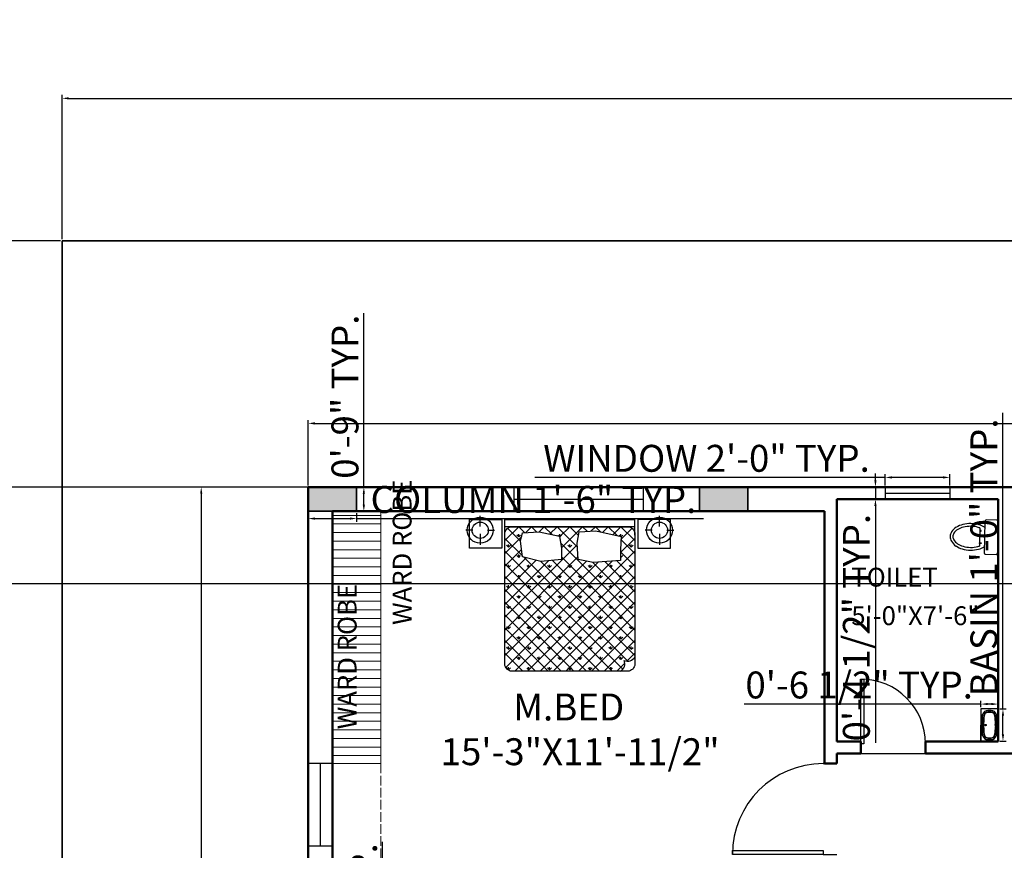
# Model space of a CAD drawing. Units: inches. Extents: x 2214 to 3937, y 762 to 2085.
# Tile 4 of 9: x 2567 to 2933, y 1777 to 2085. Entities that reach past the tile are written whole.
import ezdxf

# ---------------------------------------------------------------- set-up
doc = ezdxf.new("R2010")
doc.units = ezdxf.units.IN
doc.linetypes.add('ACAD_ISO02W100', pattern=[15, 12, -3])
for name, color, linetype, lineweight in [('A-ANNO-DIMS', 2, 'Continuous', 18), ('A-ANNO-TEXT', 7, 'Continuous', 18), ('A-AREA-IDEN', 7, 'Continuous', 25), ('A-CASE-OVHD', 252, 'ACAD_ISO02W100', 13), ('A-CASE-PATT', 252, 'Continuous', 13), ('A-COLS', 5, 'Continuous', 35), ('A-FLOR-FIXT', 9, 'Continuous', 18), ('A-FURN', 8, 'Continuous', 18), ('C-ANNO-DIMS', 2, 'Continuous', 18), ('C-PROP', 3, 'Continuous', 35), ('door', 122, 'Continuous', 25), ('wall', 20, 'Continuous', 50), ('wardrobe', 252, 'Continuous', 18), ('window', 4, 'Continuous', 25)]:
    doc.layers.add(name, color=color, linetype=linetype, lineweight=lineweight)
for name, color, linetype in [('GIUONG', 70, 'Continuous'), ('NOI THAT', 42, 'Continuous'), ('THIET-BI', 21, 'Continuous')]:
    doc.layers.add(name, color=color, linetype=linetype)
doc.styles.get("Standard").update_dxf_attribs({"font": 'arial.ttf'})
doc.dimstyles.new('ISO-25', dxfattribs={"dimtxt": 10, "dimasz": 2.5, "dimexe": 1.25, "dimexo": 0.625, "dimtad": 1, "dimdec": 1, "dimlunit": 4, "dimtxsty": 'Standard', "dimcen": 2.5, "dimadec": 0, "dimazin": 0, "dimtfac": 1, "dimtdec": 1, "dimtmove": 0, "dimatfit": 3, "dimfxl": 1, "dimarcsym": 0})

# ---------------------------------------------------------------- blocks, each defined once
blk = doc.blocks.new('*U2')
for p, q in [((0, 0), (0, -6)), ((40, 0), (40, -6))]:
    blk.add_line(p, q)
blk.add_lwpolyline([(0, 0), (0, 40), (1.75, 40), (1.75, 0)], close=True)
blk.add_arc((0, 0), 40, 0, 90)
blk = doc.blocks.new('*X8')
at = {"color": 0}
for p, q in [((0, 0), (0, 0)), ((-707, -141), (-734, -115)), ((-707, -141), (-707, -104)), ((-707, -141), (-681, -115)), ((-566, 0), (-566, 0)), ((-566, 0), (-566, 0)), ((-283, 0), (-283, 0)), ((-283, 0), (-283, 0)), ((-156, -126), (-168, -115)), ((-141, -141), (-141, -104)), ((-141, -141), (-115, -115)), ((120, -120), (115, -115)), ((283, 0), (283, 0)), ((566, 0), (566, 0)), ((699, -134), (681, -115)), ((707, -135), (707, -104)), ((710, -139), (734, -115)), ((-849, -283), (-875, -256)), ((-849, -283), (-849, -245)), ((-849, -283), (-822, -256)), ((-141, -141), (-142, -140)), ((0, -283), (-27, -256)), ((0, -283), (0, -245)), ((0, -283), (27, -256)), ((849, -283), (822, -256)), ((849, -283), (849, -245)), ((849, -283), (875, -256)), ((-707, -424), (-734, -398)), ((-707, -424), (-707, -387)), ((-707, -424), (-681, -398)), ((-116, -399), (-115, -398)), ((707, -424), (707, -387)), ((707, -424), (734, -398)), ((-849, -566), (-875, -539)), ((-849, -566), (-849, -528)), ((-849, -566), (-822, -539)), ((-566, -566), (-592, -539)), ((-566, -566), (-566, -528)), ((-566, -566), (-539, -539)), ((-283, -566), (-309, -539)), ((-283, -566), (-283, -528)), ((-283, -566), (-256, -539)), ((0, -566), (-27, -539)), ((0, -566), (0, -528)), ((0, -566), (27, -539)), ((283, -566), (256, -539)), ((283, -566), (283, -528)), ((283, -566), (309, -539)), ((566, -566), (539, -539)), ((566, -566), (566, -528)), ((566, -566), (592, -539)), ((707, -424), (703, -420)), ((849, -566), (822, -539)), ((849, -566), (849, -528)), ((849, -566), (875, -539)), ((-707, -707), (-734, -681)), ((-707, -707), (-707, -670)), ((-707, -707), (-681, -681)), ((-424, -707), (-451, -681)), ((-424, -707), (-424, -670)), ((-424, -707), (-398, -681)), ((-141, -707), (-168, -681)), ((-141, -707), (-141, -670)), ((-141, -707), (-115, -681)), ((141, -707), (115, -681)), ((141, -707), (141, -670)), ((141, -707), (168, -681)), ((424, -707), (398, -681)), ((424, -707), (424, -670)), ((424, -707), (451, -681)), ((707, -707), (681, -681)), ((707, -707), (707, -670)), ((707, -707), (734, -681)), ((-849, -849), (-849, -811)), ((-566, -849), (-566, -811)), ((-283, -849), (-283, -811)), ((0, -849), (0, -811)), ((283, -849), (283, -811)), ((566, -849), (566, -811)), ((849, -849), (849, -811)), ((-849, -849), (-875, -822)), ((-849, -849), (-822, -822)), ((-707, -990), (-707, -952)), ((-566, -849), (-592, -822)), ((-566, -849), (-539, -822)), ((-424, -990), (-424, -952)), ((-283, -849), (-309, -822)), ((-283, -849), (-256, -822)), ((-141, -990), (-141, -952)), ((0, -849), (-27, -822)), ((0, -849), (27, -822)), ((141, -990), (141, -952)), ((283, -849), (256, -822)), ((283, -849), (309, -822)), ((424, -990), (424, -952)), ((566, -849), (539, -822)), ((566, -849), (592, -822)), ((707, -990), (707, -952)), ((849, -849), (822, -822)), ((849, -849), (875, -822)), ((-707, -990), (-734, -963)), ((-707, -990), (-681, -963)), ((-424, -990), (-451, -963)), ((-424, -990), (-398, -963)), ((-141, -990), (-168, -963)), ((-141, -990), (-115, -963)), ((141, -990), (115, -963)), ((141, -990), (168, -963)), ((424, -990), (398, -963)), ((424, -990), (451, -963)), ((707, -990), (681, -963)), ((707, -990), (734, -963)), ((-849, -1131), (-875, -1105)), ((-849, -1131), (-849, -1094)), ((-849, -1131), (-822, -1105)), ((-566, -1131), (-592, -1105)), ((-566, -1131), (-566, -1094)), ((-566, -1131), (-539, -1105)), ((-283, -1131), (-309, -1105)), ((-283, -1131), (-283, -1094)), ((-283, -1131), (-256, -1105)), ((0, -1131), (-27, -1105)), ((0, -1131), (0, -1094)), ((0, -1131), (27, -1105)), ((283, -1131), (256, -1105)), ((283, -1131), (283, -1094)), ((283, -1131), (309, -1105)), ((566, -1131), (539, -1105)), ((566, -1131), (566, -1094)), ((566, -1131), (592, -1105)), ((849, -1131), (822, -1105)), ((849, -1131), (849, -1094)), ((849, -1131), (875, -1105)), ((-707, -1273), (-734, -1246)), ((-707, -1273), (-707, -1235)), ((-707, -1273), (-681, -1246)), ((-424, -1273), (-451, -1246)), ((-424, -1273), (-424, -1235)), ((-424, -1273), (-398, -1246)), ((-141, -1273), (-168, -1246)), ((-141, -1273), (-141, -1235)), ((-141, -1273), (-115, -1246)), ((141, -1273), (115, -1246)), ((141, -1273), (141, -1235)), ((141, -1273), (168, -1246)), ((424, -1273), (398, -1246)), ((424, -1273), (424, -1235)), ((424, -1273), (451, -1246)), ((707, -1273), (681, -1246)), ((707, -1273), (707, -1235)), ((707, -1273), (734, -1246)), ((-849, -1414), (-875, -1388)), ((-849, -1414), (-849, -1377)), ((-849, -1414), (-822, -1388)), ((-566, -1414), (-592, -1388)), ((-566, -1414), (-566, -1377)), ((-566, -1414), (-539, -1388)), ((-283, -1414), (-309, -1388)), ((-283, -1414), (-283, -1377)), ((-283, -1414), (-256, -1388)), ((0, -1414), (-27, -1388)), ((0, -1414), (0, -1377)), ((0, -1414), (27, -1388)), ((283, -1414), (256, -1388)), ((283, -1414), (283, -1377)), ((283, -1414), (309, -1388)), ((566, -1414), (539, -1388)), ((566, -1414), (566, -1377)), ((566, -1414), (592, -1388)), ((849, -1414), (822, -1388)), ((849, -1414), (849, -1377)), ((849, -1414), (875, -1388)), ((-707, -1556), (-734, -1529)), ((-707, -1556), (-707, -1518)), ((-707, -1556), (-681, -1529)), ((-424, -1556), (-451, -1529)), ((-424, -1556), (-424, -1518)), ((-424, -1556), (-398, -1529)), ((-141, -1556), (-168, -1529)), ((-141, -1556), (-141, -1518)), ((-141, -1556), (-115, -1529)), ((141, -1556), (115, -1529)), ((141, -1556), (141, -1518)), ((141, -1556), (168, -1529)), ((424, -1556), (398, -1529)), ((424, -1556), (424, -1518)), ((424, -1556), (451, -1529)), ((707, -1556), (681, -1529)), ((707, -1556), (707, -1518)), ((707, -1556), (734, -1529)), ((-849, -1697), (-875, -1671)), ((-849, -1697), (-849, -1660)), ((-849, -1697), (-822, -1671)), ((-566, -1697), (-592, -1671)), ((-566, -1697), (-566, -1660)), ((-566, -1697), (-539, -1671)), ((-283, -1697), (-309, -1671)), ((-283, -1697), (-283, -1660)), ((-283, -1697), (-256, -1671)), ((0, -1697), (-27, -1671)), ((0, -1697), (0, -1660)), ((0, -1697), (27, -1671)), ((283, -1697), (256, -1671)), ((283, -1697), (283, -1660)), ((283, -1697), (309, -1671)), ((566, -1697), (539, -1671)), ((566, -1697), (566, -1660)), ((566, -1697), (592, -1671)), ((849, -1697), (822, -1671)), ((849, -1697), (849, -1660)), ((849, -1697), (875, -1671)), ((-707, -1838), (-734, -1812)), ((-707, -1838), (-707, -1801)), ((-707, -1838), (-681, -1812)), ((-424, -1838), (-451, -1812)), ((-424, -1838), (-424, -1801)), ((-424, -1838), (-398, -1812)), ((-141, -1838), (-168, -1812)), ((-141, -1838), (-141, -1801)), ((-141, -1838), (-115, -1812)), ((141, -1838), (115, -1812)), ((141, -1838), (141, -1801)), ((141, -1838), (168, -1812)), ((424, -1838), (398, -1812)), ((424, -1838), (424, -1801)), ((424, -1838), (451, -1812)), ((707, -1838), (681, -1812)), ((707, -1838), (707, -1801)), ((707, -1838), (734, -1812)), ((-849, -1980), (-875, -1953)), ((-849, -1980), (-849, -1942)), ((-849, -1980), (-822, -1953)), ((-566, -1980), (-592, -1953)), ((-566, -1980), (-566, -1942)), ((-566, -1980), (-539, -1953)), ((-283, -1980), (-309, -1953)), ((-283, -1980), (-283, -1942)), ((-283, -1980), (-256, -1953)), ((0, -1980), (-27, -1953)), ((0, -1980), (0, -1942)), ((0, -1980), (27, -1953)), ((283, -1980), (256, -1953)), ((283, -1980), (283, -1942)), ((283, -1980), (309, -1953)), ((566, -1980), (539, -1953)), ((566, -1980), (566, -1942)), ((566, -1980), (592, -1953))]:
    blk.add_line(p, q, dxfattribs=at)
blk = doc.blocks.new('*X7')
at = {"color": 0}
for p, q in [((-900, -193), (-707, 0)), ((-623, -84), (-707, 0)), ((-614, -83), (-530, 0)), ((-457, -74), (-530, 0)), ((-425, -72), (-354, 0)), ((-245, -108), (-354, 0)), ((-278, -101), (-177, 0)), ((103, -280), (-177, 0)), ((-142, -142), (0, 0)), ((-117, -294), (177, 0)), ((120, -120), (0, 0)), ((241, -64), (177, 0)), ((292, -61), (354, 0)), ((426, -72), (354, 0)), ((452, -78), (530, 0)), ((654, -123), (530, 0)), ((596, -111), (707, 0)), ((900, -193), (707, 0)), ((-683, -201), (-862, -22)), ((708, -175), (862, -22)), ((-900, -370), (-667, -137)), ((-656, -405), (-900, -161)), ((-900, -1254), (101, -252)), ((900, -1254), (-128, -225)), ((703, -358), (900, -161)), ((900, -370), (708, -178)), ((-900, -546), (-668, -314)), ((735, -1973), (-900, -337)), ((-763, -2000), (900, -337)), ((900, -546), (703, -349)), ((-900, -1430), (112, -418)), ((-900, -723), (-605, -429)), ((-900, -900), (-465, -465)), ((-900, -1077), (-293, -470)), ((-900, -1607), (231, -476)), ((-900, -1784), (394, -489)), ((586, -2000), (-900, -514)), ((-888, -1948), (586, -475)), ((801, -1862), (-641, -419)), ((-586, -2000), (900, -514)), ((900, -1784), (-404, -480)), ((900, -1607), (-243, -465)), ((900, -1430), (-116, -415)), ((900, -1077), (317, -494)), ((900, -900), (483, -483)), ((900, -723), (647, -470)), ((409, -2000), (-900, -691)), ((-409, -2000), (900, -691)), ((232, -2000), (-900, -868)), ((-232, -2000), (900, -868)), ((55, -2000), (-900, -1045)), ((-55, -2000), (900, -1045)), ((-121, -2000), (-900, -1221)), ((121, -2000), (900, -1221)), ((-298, -2000), (-900, -1398)), ((298, -2000), (900, -1398)), ((-475, -2000), (-900, -1575)), ((475, -2000), (900, -1575)), ((-652, -2000), (-900, -1752)), ((790, -1861), (900, -1752)), ((652, -2000), (761, -1890)), ((-835, -1994), (-894, -1935))]:
    blk.add_line(p, q, dxfattribs=at)
blk = doc.blocks.new('A$C190D2546')
at = {"layer": 'GIUONG'}
for points in [[(787, 1584), (758, 1799), (787, 1914), (1016, 1928), (1296, 1871), (1325, 1699), (1325, 1548), (1038, 1519)], [(1555, 1548), (1541, 1771), (1569, 1928), (1799, 1943), (2151, 1864), (2144, 1685), (2144, 1534), (1763, 1505)]]:
    blk.add_lwpolyline(points, close=True, dxfattribs=at)
for centre, radius in [((200, 1951), 180), ((200, 1951), 112), ((2682, 1951), 180), ((2682, 1951), 112)]:
    blk.add_circle(centre, radius, dxfattribs=at)
at = {"layer": 'NOI THAT'}
for p, q in [((200, 2001), (200, 2151)), ((541, 2100), (2341, 2100)), ((541, 1881), (541, 2100)), ((2341, 1881), (2341, 2100)), ((2682, 2001), (2682, 2151)), ((100, 1951), (0, 1951)), ((300, 1951), (400, 1951)), ((2341, 2000), (541, 2000)), ((2582, 1951), (2482, 1951)), ((2782, 1951), (2882, 1951)), ((200, 1901), (200, 1751)), ((2682, 1901), (2682, 1751))]:
    blk.add_line(p, q, dxfattribs=at)
for points in [[(500, 2101), (500, 1701), (50, 1701), (50, 2101)], [(2382, 2101), (2382, 1701), (2832, 1701), (2832, 2101)]]:
    blk.add_lwpolyline(points, close=True, dxfattribs=at)
blk.add_lwpolyline([(641, 2000), (2241, 2000, -0.414214), (2341, 1900), (2341, 100, -0.414214), (2241, 0), (641, 0, -0.414214), (541, 100), (541, 1900, -0.414214)], format="xyb", close=True, dxfattribs=at)
for centre, start, end in [((2091, 100), 296.5651, 26.5651), ((2241, 250), 243.4349, 333.4349)]:
    blk.add_arc(centre, 112, start, end, dxfattribs=at)
for name in ['*X7', '*X8']:
    blk.add_blockref(name, (1441, 2000), dxfattribs=at)
blk = doc.blocks.new('A$C65B13726')
at = {"layer": 'THIET-BI'}
for p, q in [((0, 400), (0, 200)), ((0, 400), (375, 400)), ((134, 362), (621, 360)), ((375, 291), (357, 291)), ((357, 291), (393, 291)), ((375, 291), (375, 309)), ((375, 309), (375, 274)), ((134, 39), (616, 39))]:
    blk.add_line(p, q, dxfattribs=at)
blk.add_lwpolyline([(0, 400), (0, 0), (750, 0), (750, 400)], close=True, dxfattribs=at)
blk.add_lwpolyline([(714, 200), (714, 240, 0.341607), (621, 360), (598, 366, 0.001439), (593, 367, 0.035276), (375, 382, 0.035276), (157, 367, 0.001439), (152, 366), (129, 360, 0.341607), (36, 240), (36, 200), (36, 161, 0.341607), (129, 40), (152, 34, 0.001439), (157, 33, 0.035276), (375, 18, 0.035276), (593, 33, 0.001439), (598, 34), (621, 40, 0.341607), (714, 161)], format="xyb", close=True, dxfattribs=at)
for points in [[(323, 348, 0.026733), (162, 334, 0.000876), (159, 333), (137, 327, 0.341782), (70, 240), (70, 161, 0.341782), (137, 73), (159, 67, 0.000876), (162, 67, 0.026747), (323, 52, 0.035276)], [(337, 337, 0.028876), (163, 323, 0.00069), (161, 322), (140, 317, 0.341861), (81, 240), (81, 160, 0.341861), (140, 83), (161, 78, 0.00069), (163, 77, 0.028898), (337, 63, 0.035276)], [(407, 348, 0.00526), (375, 349, 0.005313), (343, 348, 0.000876)], [(394, 338, 0.003179), (375, 338, 0.003179), (356, 338, 0.00069)], [(375, 382), (375, 382, 0.025118)], [(375, 382), (375, 382, 0.035276)], [(669, 200), (669, 240, 0.341861), (610, 317), (589, 322, 0.00069), (587, 323, 0.028876), (413, 337, 0.003179)], [(680, 200), (680, 240, 0.341782), (613, 327), (591, 333, 0.000876), (588, 334, 0.026733), (427, 348, 0.006503)], [(343, 52, 0.005316), (375, 52, 0.005263), (407, 52, 0.000876)], [(356, 62, 0.003135), (375, 62, 0.003135), (394, 62, 0.00069)], [(375, 17), (375, 17, 0.035276)], [(413, 63, 0.028961), (587, 77, 0.00069), (589, 78), (610, 83, 0.341861), (669, 160), (669, 200)], [(427, 52, 0.026747), (588, 67, 0.000876), (591, 67), (613, 73, 0.341782), (680, 161), (680, 200)]]:
    blk.add_lwpolyline(points, format="xyb", dxfattribs=at)
blk.add_circle((375, 291), 14.5, dxfattribs=at)
for centre, radius, start, end in [((375, 400), 73.6, 211.9576, 327.7237), ((324, 352), 19.1, 310.8832, 28.9258), ((375, 400), 65.2, 239.0852, 300.5961), ((426, 351), 19.1, 150.7555, 228.798), ((375, 0), 73.6, 32.2763, 148.0424), ((324, 48), 19.1, 331.0742, 49.1168), ((375, 0), 65.2, 59.4039, 120.9148), ((426, 49), 19.1, 131.202, 209.2445)]:
    blk.add_arc(centre, radius, start, end, dxfattribs=at)
blk = doc.blocks.new('A$C5AF77858')
at = {"layer": 'THIET-BI'}
for p, q in [((0, 675), (0, 525)), ((475, 700), (25, 700)), ((500, 525), (500, 675)), ((25, 500), (475, 500)), ((154, 452), (154, 430)), ((164, 452), (154, 452)), ((164, 430), (164, 452)), ((336, 430), (336, 452)), ((336, 452), (346, 452)), ((346, 452), (346, 430)), ((117, 430), (383, 430)), ((154, 430), (164, 430)), ((346, 430), (336, 430))]:
    blk.add_line(p, q, dxfattribs=at)
for centre, radius, start, end in [((25, 675), 25, 90, 180), ((475, 675), 25, 0, 90), ((25, 525), 25, 180, 270), ((384, 334), 323, 149.0966, 164.9269), ((116, 334), 323, 15.0731, 30.9034), ((475, 525), 25, 270, 0), ((514, 299), 458, 164.9269, 180), ((514, 299), 458, 180, 195.0731), ((514, 299), 418, 164.9269, 180), ((514, 299), 418, 180, 195.0731), ((384, 334), 283, 160.176, 164.9269), ((116, 334), 283, 15.0731, 19.824), ((-14, 299), 418, 0, 15.0731), ((-14, 299), 418, 344.9269, 0), ((-14, 299), 458, 0, 15.0731), ((-14, 299), 458, 344.9269, 0), ((384, 264), 323, 195.0731, 213.0315), ((384, 264), 283, 195.0731, 213.0315), ((116, 264), 283, 326.9685, 344.9269), ((116, 264), 323, 326.9685, 344.9269), ((302, 210), 226, 213.0315, 237.5002), ((302, 210), 186, 213.0315, 237.5002), ((250, 129), 129, 237.5002, 270), ((250, 129), 89.3, 237.5002, 270), ((250, 129), 89.3, 270, 302.4998), ((250, 129), 129, 270, 302.4998), ((198, 210), 186, 302.4998, 326.9685), ((198, 210), 226, 302.4998, 326.9685)]:
    blk.add_arc(centre, radius, start, end, dxfattribs=at)
blk = doc.blocks.new('*D18')
at = {"layer": 'A-ANNO-DIMS', "color": 0, "lineweight": -2, "ltscale": 0.3, "transparency": 16777216}
for p, q in [((2673.43, 1911.72), (2633.05, 1911.72)), ((2634.3, 1909.22), (2634.3, 1477.72)), ((2673.43, 1475.22), (2633.05, 1475.22))]:
    blk.add_line(p, q, dxfattribs=at)
at = {"layer": 'A-ANNO-DIMS', "color": 0, "ltscale": 0.3, "transparency": 16777216}
for points in [[(2633.89, 1909.22), (2634.72, 1909.22), (2634.3, 1911.72)], [(2633.89, 1477.72), (2634.72, 1477.72), (2634.3, 1475.22)]]:
    blk.add_solid(points, dxfattribs=at)
at = {"layer": 'Defpoints', "color": 0, "ltscale": 0.3, "transparency": 16777216}
for p in [(2674.06, 1911.72), (2634.3, 1475.22), (2674.06, 1475.22)]:
    blk.add_point(p, dxfattribs=at)
at = {"layer": 'A-ANNO-DIMS', "color": 0, "ltscale": 0.3, "transparency": 16777216, "insert": (2605.37, 1693.47), "char_height": 24, "attachment_point": 5, "rotation": 90}
blk.add_mtext('36\'-4{\\H1x;\\S1/2;}"', dxfattribs=at)
blk = doc.blocks.new('*D19')
at = {"layer": 'C-ANNO-DIMS', "color": 0, "lineweight": -2, "ltscale": 0.3, "transparency": 16777216}
for p, q in [((2582.56, 2003.84), (2582.56, 2057.46)), ((3662.56, 2003.84), (3662.56, 2057.46)), ((2585.06, 2056.21), (3660.06, 2056.21))]:
    blk.add_line(p, q, dxfattribs=at)
at = {"layer": 'C-ANNO-DIMS', "color": 0, "ltscale": 0.3, "transparency": 16777216}
for points in [[(2585.06, 2056.63), (2585.06, 2055.8), (2582.56, 2056.21)], [(3660.06, 2056.63), (3660.06, 2055.8), (3662.56, 2056.21)]]:
    blk.add_solid(points, dxfattribs=at)
at = {"layer": 'Defpoints', "color": 0, "ltscale": 0.3, "transparency": 16777216}
for p in [(3662.56, 2056.21), (2582.56, 2003.22), (3662.56, 2003.22)]:
    blk.add_point(p, dxfattribs=at)
at = {"layer": 'C-ANNO-DIMS', "color": 0, "ltscale": 0.3, "transparency": 16777216, "insert": (3122.56, 2069.09), "char_height": 24, "attachment_point": 5}
blk.add_mtext("90'", dxfattribs=at)
blk = doc.blocks.new('*D20')
at = {"layer": 'C-ANNO-DIMS', "color": 0, "lineweight": -2, "ltscale": 0.3, "transparency": 16777216}
for p, q in [((2581.93, 2003.22), (2545.31, 2003.22)), ((2546.56, 2000.72), (2546.56, 1357.72)), ((2581.93, 1355.22), (2545.31, 1355.22))]:
    blk.add_line(p, q, dxfattribs=at)
at = {"layer": 'C-ANNO-DIMS', "color": 0, "ltscale": 0.3, "transparency": 16777216}
for points in [[(2546.14, 2000.72), (2546.97, 2000.72), (2546.56, 2003.22)], [(2546.14, 1357.72), (2546.97, 1357.72), (2546.56, 1355.22)]]:
    blk.add_solid(points, dxfattribs=at)
at = {"layer": 'Defpoints', "color": 0, "ltscale": 0.3, "transparency": 16777216}
for p in [(2582.56, 2003.22), (2546.56, 1355.22), (2582.56, 1355.22)]:
    blk.add_point(p, dxfattribs=at)
at = {"layer": 'C-ANNO-DIMS', "color": 0, "ltscale": 0.3, "transparency": 16777216, "insert": (2533.73, 1679.22), "char_height": 24, "attachment_point": 5, "rotation": 90}
blk.add_mtext("54'", dxfattribs=at)
blk = doc.blocks.new('*D25')
at = {"layer": 'A-ANNO-DIMS', "color": 0, "lineweight": -2, "ltscale": 0.3, "transparency": 16777216}
for p, q in [((2674.06, 1912.34), (2674.06, 1936.65)), ((3571.06, 1912.34), (3571.06, 1936.65)), ((2676.56, 1935.4), (3568.56, 1935.4))]:
    blk.add_line(p, q, dxfattribs=at)
at = {"layer": 'A-ANNO-DIMS', "color": 0, "ltscale": 0.3, "transparency": 16777216}
for points in [[(2676.56, 1935.82), (2676.56, 1934.98), (2674.06, 1935.4)], [(3568.56, 1935.82), (3568.56, 1934.98), (3571.06, 1935.4)]]:
    blk.add_solid(points, dxfattribs=at)
at = {"layer": 'Defpoints', "color": 0, "ltscale": 0.3, "transparency": 16777216}
for p in [(3571.06, 1935.4), (2674.06, 1911.72), (3571.06, 1911.72)]:
    blk.add_point(p, dxfattribs=at)
at = {"layer": 'A-ANNO-DIMS', "color": 0, "ltscale": 0.3, "transparency": 16777216, "insert": (3122.56, 1948.28), "char_height": 24, "attachment_point": 5}
blk.add_mtext('74\'-9"', dxfattribs=at)
blk = doc.blocks.new('COL-18X9')
at = {"ltscale": 0.3}
h = blk.add_hatch(color=256, dxfattribs=at)
h.dxf.hatch_style = 1
h.paths.add_polyline_path([(18, 0), (18, 9), (0, 9), (0, 0)])
blk.add_lwpolyline([(0, 9), (18, 9), (18, 0), (0, 0)], close=True, dxfattribs=at)
blk = doc.blocks.new('WIN-48X9')
for p, q in [((0, 48), (9, 48)), ((0, 0), (9, 0))]:
    blk.add_line(p, q)
at = {"ltscale": 0.3}
blk.add_line((4.5, 0), (4.5, 48), dxfattribs=at)
blk = doc.blocks.new('WIN-24X4_5')
for p, q in [((0, 0), (0, 4.5)), ((24, 0), (24, 4.5))]:
    blk.add_line(p, q)
at = {"ltscale": 0.3}
blk.add_line((24, 2.25), (0, 2.25), dxfattribs=at)
blk = doc.blocks.new('*D35')
at = {"layer": 'C-ANNO-DIMS', "color": 0, "lineweight": -2, "ltscale": 0.3, "transparency": 16777216}
for p, q in [((2674.06, 1902.09), (2674.06, 1898.77)), ((2676.56, 1900.02), (2689.56, 1900.02)), ((2692.06, 1902.09), (2692.06, 1898.77)), ((2692.06, 1900.02), (2821.07, 1900.02))]:
    blk.add_line(p, q, dxfattribs=at)
at = {"layer": 'C-ANNO-DIMS', "color": 0, "ltscale": 0.3, "transparency": 16777216}
for points in [[(2676.56, 1900.44), (2676.56, 1899.6), (2674.06, 1900.02)], [(2689.56, 1900.44), (2689.56, 1899.6), (2692.06, 1900.02)]]:
    blk.add_solid(points, dxfattribs=at)
at = {"layer": 'Defpoints', "color": 0, "ltscale": 0.3, "transparency": 16777216}
for p in [(2674.06, 1902.72), (2692.06, 1902.72), (2692.06, 1900.02)]:
    blk.add_point(p, dxfattribs=at)
at = {"layer": 'C-ANNO-DIMS', "color": 0, "ltscale": 0.3, "transparency": 16777216, "insert": (2757.81, 1905.82), "char_height": 10, "attachment_point": 5}
blk.add_mtext('COLUMN 1\'-6" TYP.', dxfattribs=at)
blk = doc.blocks.new('*D36')
at = {"layer": 'C-ANNO-DIMS', "color": 0, "lineweight": -2, "ltscale": 0.3, "transparency": 16777216}
for p, q in [((2694.76, 1911.72), (2694.76, 1976.42)), ((2692.68, 1911.72), (2696.01, 1911.72)), ((2694.76, 1905.22), (2694.76, 1909.22)), ((2692.68, 1902.72), (2696.01, 1902.72))]:
    blk.add_line(p, q, dxfattribs=at)
at = {"layer": 'C-ANNO-DIMS', "color": 0, "ltscale": 0.3, "transparency": 16777216}
for points in [[(2694.34, 1909.22), (2695.17, 1909.22), (2694.76, 1911.72)], [(2694.34, 1905.22), (2695.17, 1905.22), (2694.76, 1902.72)]]:
    blk.add_solid(points, dxfattribs=at)
at = {"layer": 'Defpoints', "color": 0, "ltscale": 0.3, "transparency": 16777216}
for p in [(2692.06, 1911.72), (2694.76, 1911.72), (2692.06, 1902.72)]:
    blk.add_point(p, dxfattribs=at)
at = {"layer": 'C-ANNO-DIMS', "color": 0, "ltscale": 0.3, "transparency": 16777216, "insert": (2689.03, 1945.32), "char_height": 10, "attachment_point": 5, "rotation": 90}
blk.add_mtext('0\'-9" TYP.', dxfattribs=at)
blk = doc.blocks.new('*D38')
at = {"layer": 'C-ANNO-DIMS', "color": 0, "lineweight": -2, "ltscale": 0.3, "transparency": 16777216}
for p, q in [((2701.66, 1715.22), (2701.66, 1779.92)), ((2698.68, 1715.22), (2702.91, 1715.22)), ((2701.66, 1708.72), (2701.66, 1712.72)), ((2698.68, 1706.22), (2702.91, 1706.22))]:
    blk.add_line(p, q, dxfattribs=at)
at = {"layer": 'C-ANNO-DIMS', "color": 0, "ltscale": 0.3, "transparency": 16777216}
for points in [[(2701.24, 1712.72), (2702.07, 1712.72), (2701.66, 1715.22)], [(2701.24, 1708.72), (2702.07, 1708.72), (2701.66, 1706.22)]]:
    blk.add_solid(points, dxfattribs=at)
at = {"layer": 'Defpoints', "color": 0, "ltscale": 0.3, "transparency": 16777216}
for p in [(2698.06, 1715.22), (2701.66, 1715.22), (2698.06, 1706.22)]:
    blk.add_point(p, dxfattribs=at)
at = {"layer": 'C-ANNO-DIMS', "color": 0, "ltscale": 0.3, "transparency": 16777216, "insert": (2695.93, 1748.82), "char_height": 10, "attachment_point": 5, "rotation": 90}
blk.add_mtext('0\'-9" TYP.', dxfattribs=at)
blk = doc.blocks.new('*D43')
at = {"layer": 'C-ANNO-DIMS', "color": 0, "lineweight": -2, "ltscale": 0.3, "transparency": 16777216}
for p, q in [((2888.56, 1915.32), (2758.27, 1915.32)), ((2888.56, 1912.34), (2888.56, 1916.57)), ((2910.06, 1915.32), (2891.06, 1915.32)), ((2912.56, 1912.34), (2912.56, 1916.57))]:
    blk.add_line(p, q, dxfattribs=at)
at = {"layer": 'C-ANNO-DIMS', "color": 0, "ltscale": 0.3, "transparency": 16777216}
for points in [[(2891.06, 1915.74), (2891.06, 1914.9), (2888.56, 1915.32)], [(2910.06, 1915.74), (2910.06, 1914.9), (2912.56, 1915.32)]]:
    blk.add_solid(points, dxfattribs=at)
at = {"layer": 'Defpoints', "color": 0, "ltscale": 0.3, "transparency": 16777216}
for p in [(2888.56, 1915.32), (2888.56, 1911.72), (2912.56, 1911.72)]:
    blk.add_point(p, dxfattribs=at)
at = {"layer": 'C-ANNO-DIMS', "color": 0, "ltscale": 0.3, "transparency": 16777216, "insert": (2822.16, 1921.12), "char_height": 10, "attachment_point": 5}
blk.add_mtext('WINDOW 2\'-0" TYP.', dxfattribs=at)
blk = doc.blocks.new('*D44')
at = {"layer": 'C-ANNO-DIMS', "color": 0, "lineweight": -2, "ltscale": 0.3, "transparency": 16777216}
for p, q in [((2884.96, 1914.22), (2884.96, 1916.72)), ((2887.93, 1911.72), (2883.71, 1911.72)), ((2884.96, 1911.72), (2884.96, 1907.22)), ((2887.93, 1907.22), (2883.71, 1907.22)), ((2884.96, 1904.72), (2884.96, 1816.71))]:
    blk.add_line(p, q, dxfattribs=at)
at = {"layer": 'C-ANNO-DIMS', "color": 0, "ltscale": 0.3, "transparency": 16777216}
for points in [[(2884.54, 1914.22), (2885.37, 1914.22), (2884.96, 1911.72)], [(2884.54, 1904.72), (2885.37, 1904.72), (2884.96, 1907.22)]]:
    blk.add_solid(points, dxfattribs=at)
at = {"layer": 'Defpoints', "color": 0, "ltscale": 0.3, "transparency": 16777216}
for p in [(2888.56, 1911.72), (2884.96, 1907.22), (2888.56, 1907.22)]:
    blk.add_point(p, dxfattribs=at)
at = {"layer": 'C-ANNO-DIMS', "color": 0, "ltscale": 0.3, "transparency": 16777216, "insert": (2879.16, 1859.47), "char_height": 10, "attachment_point": 5, "rotation": 90}
blk.add_mtext('0\'-4 1/2" TYP.', dxfattribs=at)
blk = doc.blocks.new('*D47')
at = {"layer": 'C-ANNO-DIMS', "color": 0, "lineweight": -2, "ltscale": 0.3, "transparency": 16777216}
for p, q in [((2932.36, 1829.27), (2932.36, 1939.34)), ((2931.18, 1829.27), (2933.61, 1829.27)), ((2932.36, 1819.77), (2932.36, 1826.77)), ((2931.18, 1817.27), (2933.61, 1817.27))]:
    blk.add_line(p, q, dxfattribs=at)
at = {"layer": 'C-ANNO-DIMS', "color": 0, "ltscale": 0.3, "transparency": 16777216}
for points in [[(2931.94, 1826.77), (2932.77, 1826.77), (2932.36, 1829.27)], [(2931.94, 1819.77), (2932.77, 1819.77), (2932.36, 1817.27)]]:
    blk.add_solid(points, dxfattribs=at)
at = {"layer": 'Defpoints', "color": 0, "ltscale": 0.3, "transparency": 16777216}
for p in [(2930.56, 1829.27), (2932.36, 1829.27), (2930.56, 1817.27)]:
    blk.add_point(p, dxfattribs=at)
at = {"layer": 'C-ANNO-DIMS', "color": 0, "ltscale": 0.3, "transparency": 16777216, "insert": (2926.56, 1885.56), "char_height": 10, "attachment_point": 5, "rotation": 90}
blk.add_mtext('BASIN 1\'-0" TYP.', dxfattribs=at)
blk = doc.blocks.new('*D48')
at = {"layer": 'C-ANNO-DIMS', "color": 0, "lineweight": -2, "ltscale": 0.3, "transparency": 16777216}
for p, q in [((2924.16, 1831.07), (2836.15, 1831.07)), ((2924.16, 1829.9), (2924.16, 1832.32)), ((2928.06, 1831.07), (2926.66, 1831.07)), ((2930.56, 1829.9), (2930.56, 1832.32))]:
    blk.add_line(p, q, dxfattribs=at)
at = {"layer": 'C-ANNO-DIMS', "color": 0, "ltscale": 0.3, "transparency": 16777216}
for points in [[(2926.66, 1831.49), (2926.66, 1830.66), (2924.16, 1831.07)], [(2928.06, 1831.49), (2928.06, 1830.66), (2930.56, 1831.07)]]:
    blk.add_solid(points, dxfattribs=at)
at = {"layer": 'Defpoints', "color": 0, "ltscale": 0.3, "transparency": 16777216}
for p in [(2924.16, 1831.07), (2924.16, 1829.27), (2930.56, 1829.27)]:
    blk.add_point(p, dxfattribs=at)
at = {"layer": 'C-ANNO-DIMS', "color": 0, "ltscale": 0.3, "transparency": 16777216, "insert": (2878.9, 1836.87), "char_height": 10, "attachment_point": 5}
blk.add_mtext('0\'-6 1/2" TYP.', dxfattribs=at)
blk = doc.blocks.new('*D62')
at = {"layer": 'C-ANNO-DIMS', "color": 0, "lineweight": -2, "ltscale": 0.3, "transparency": 16777216}
for p, q in [((3240.43, 1911.72), (2225.23, 1911.72)), ((2226.48, 1909.22), (2226.48, 1878.22)), ((3240.43, 1875.72), (2225.23, 1875.72))]:
    blk.add_line(p, q, dxfattribs=at)
at = {"layer": 'C-ANNO-DIMS', "color": 0, "ltscale": 0.3, "transparency": 16777216}
for points in [[(2226.07, 1909.22), (2226.9, 1909.22), (2226.48, 1911.72)], [(2226.07, 1878.22), (2226.9, 1878.22), (2226.48, 1875.72)]]:
    blk.add_solid(points, dxfattribs=at)
at = {"layer": 'Defpoints', "color": 0, "ltscale": 0.3, "transparency": 16777216}
for p in [(3241.06, 1911.72), (2226.48, 1875.72), (3241.06, 1875.72)]:
    blk.add_point(p, dxfattribs=at)
at = {"layer": 'C-ANNO-DIMS', "color": 0, "ltscale": 0.3, "transparency": 16777216, "insert": (2220.75, 1893.72), "char_height": 10, "attachment_point": 5, "rotation": 90}
blk.add_mtext('3\'-0"', dxfattribs=at)
blk = doc.blocks.new('*D63')
at = {"layer": 'C-ANNO-DIMS', "color": 0, "lineweight": -2, "ltscale": 0.3, "transparency": 16777216}
for p, q in [((3240.43, 1875.72), (2225.23, 1875.72)), ((2226.48, 1873.22), (2226.48, 1739.22)), ((3240.43, 1736.72), (2225.23, 1736.72))]:
    blk.add_line(p, q, dxfattribs=at)
at = {"layer": 'C-ANNO-DIMS', "color": 0, "ltscale": 0.3, "transparency": 16777216}
for points in [[(2226.07, 1873.22), (2226.9, 1873.22), (2226.48, 1875.72)], [(2226.07, 1739.22), (2226.9, 1739.22), (2226.48, 1736.72)]]:
    blk.add_solid(points, dxfattribs=at)
at = {"layer": 'Defpoints', "color": 0, "ltscale": 0.3, "transparency": 16777216}
for p in [(3241.06, 1875.72), (2226.48, 1736.72), (3241.06, 1736.72)]:
    blk.add_point(p, dxfattribs=at)
at = {"layer": 'C-ANNO-DIMS', "color": 0, "ltscale": 0.3, "transparency": 16777216, "insert": (2220.84, 1806.22), "char_height": 10, "attachment_point": 5, "rotation": 90}
blk.add_mtext('11\'-7"', dxfattribs=at)

msp = doc.modelspace()

# ---------------------------------------------------------------- hatches: boundary and pattern name
at = {"layer": 'A-CASE-PATT', "ltscale": 0.3}
h = msp.add_hatch(dxfattribs=at)
h.set_pattern_fill('ANSI31', color=256, scale=1.00471, angle=-45, style=0)
h.paths.add_polyline_path([(2683.06, 1808.95), (2701.06, 1808.95), (2701.06, 1902.72), (2683.06, 1902.72)])

# ---------------------------------------------------------------- linework, layer by layer
at = {"layer": 'A-CASE-OVHD', "ltscale": 0.3}
msp.add_line((2701.06, 1808.95), (2701.06, 1769.22), dxfattribs=at)
at = {"layer": 'C-PROP'}
for p, q in [((2582.56, 2003.22), (3662.56, 2003.22)), ((2582.56, 1355.22), (2582.56, 2003.22))]:
    msp.add_line(p, q, dxfattribs=at)
at = {"layer": 'door'}
msp.add_line((2879.56, 1812.72), (2903.56, 1812.72), dxfattribs=at)
at = {"layer": 'wall'}
for p, q in [((2674.06, 1911.72), (3571.06, 1911.72)), ((2674.06, 1475.22), (2674.06, 1911.72)), ((2870.56, 1907.22), (2930.56, 1907.22)), ((2870.56, 1817.22), (2870.56, 1907.22)), ((2930.56, 1817.22), (2930.56, 1907.22)), ((2683.06, 1902.72), (2866.06, 1902.72)), ((2683.06, 1769.22), (2683.06, 1902.72)), ((2866.06, 1808.95), (2866.06, 1902.72)), ((2870.56, 1817.22), (2879.56, 1817.22)), ((2879.56, 1817.22), (2879.56, 1812.72)), ((2903.56, 1817.22), (2903.56, 1812.72)), ((2903.56, 1817.22), (2930.56, 1817.22)), ((2870.56, 1812.72), (2879.56, 1812.72)), ((2870.56, 1808.95), (2870.56, 1812.72)), ((2903.56, 1812.72), (2930.56, 1812.72)), ((2930.56, 1812.72), (2995.06, 1812.72)), ((2866.06, 1808.95), (2870.56, 1808.95))]:
    msp.add_line(p, q, dxfattribs=at)
at = {"layer": 'wardrobe'}
for p, q in [((2701.06, 1902.72), (2701.06, 1808.95)), ((2701.06, 1808.95), (2683.06, 1808.95))]:
    msp.add_line(p, q, dxfattribs=at)
at = {"layer": 'window', "ltscale": 0.3}
for p, q in [((2683.06, 1808.95), (2674.06, 1808.95)), ((2678.56, 1808.95), (2678.56, 1778.22)), ((2683.06, 1778.22), (2674.06, 1778.22))]:
    msp.add_line(p, q, dxfattribs=at)

# ---------------------------------------------------------------- block references
at = {"layer": 'A-COLS'}
for p in [(2674.06, 1902.72), (2819.56, 1902.72)]:
    msp.add_blockref('COL-18X9', p, dxfattribs=at)
at = {"layer": 'A-FLOR-FIXT'}
for name, p, xscale, yscale, zscale, rotation in [('A$C5AF77858', (2912.84, 1899.72), 0.0254713121376822, 0.0254713121376822, 0.0254713121376822, 269.0249091497018), ('A$C65B13726', (2930.56, 1817.27), 0.0160009442456078, 0.0160009442456078, 0.0160009442456078, 90)]:
    msp.add_blockref(name, p, dxfattribs=dict(at, xscale=xscale, yscale=yscale, zscale=zscale, rotation=rotation))
at = {"layer": 'A-FURN', "xscale": 0.0268541596481872, "yscale": 0.0268541596481872, "zscale": 0.0268541596481872}
msp.add_blockref('A$C190D2546', (2732.65, 1843.29), dxfattribs=at)
at = {"layer": 'door', "xscale": 0.6, "yscale": 0.6, "zscale": 0.6}
msp.add_blockref('*U2', (2879.56, 1816.32), dxfattribs=at)
at = {"layer": 'door', "xscale": 0.8432138857497079, "yscale": 0.8432138857497079, "zscale": 0.8432138857497079, "rotation": 90}
msp.add_blockref('*U2', (2865.5, 1775.22), dxfattribs=at)
at = {"layer": 'window'}
for name, p, rotation in [('WIN-48X9', (2750.56, 1911.72), 270.0000000000023), ('WIN-24X4_5', (2912.56, 1911.72), 180)]:
    msp.add_blockref(name, p, dxfattribs=dict(at, rotation=rotation))

# ---------------------------------------------------------------- texts
at = {"layer": 'A-ANNO-TEXT', "ltscale": 0.3}
for p in [(2712.49, 1860.48), (2692.06, 1821.71)]:
    msp.add_text('WARD ROBE', height=7, rotation=90, dxfattribs=at).set_placement(p)
at = {"layer": 'A-AREA-IDEN', "ltscale": 0.3}
for s, height, p in [('TOILET', 7, (2875.98, 1874.74)), ('5\'-0"X7\'-6"', 7, (2875.98, 1860.41)), ('M.BED', 10, (2750.29, 1824.99)), ('15\'-3"X11\'-11/2"', 10, (2723.29, 1808.36))]:
    msp.add_text(s, height=height, dxfattribs=at).set_placement(p)

# ---------------------------------------------------------------- dimensions: what is measured, and where the dimension line sits
at = {"layer": 'A-ANNO-DIMS', "ltscale": 0.3}
dim = msp.add_linear_dim(base=(3571.06, 1935.4), p1=(2674.06, 1911.72), p2=(3571.06, 1911.72), dimstyle='ISO-25', override={"dimtxt": 24, "dimclrd": 0, "dimclre": 0, "dimclrt": 0}, dxfattribs=at)
dim.commit()
dim.dimension.update_dxf_attribs({"geometry": '*D25', "text_midpoint": (3122.56, 1948.28)})
dim = msp.add_linear_dim(base=(2634.3, 1475.22), p1=(2674.06, 1911.72), p2=(2674.06, 1475.22), angle=90, dimstyle='ISO-25', override={"dimtxt": 24, "dimclrd": 0, "dimclre": 0, "dimclrt": 0}, dxfattribs=at)
dim.commit()
dim.dimension.update_dxf_attribs({"geometry": '*D18', "text_midpoint": (2605.37, 1693.47)})
at = {"layer": 'C-ANNO-DIMS', "ltscale": 0.3}
dim = msp.add_linear_dim(base=(3662.56, 2056.21), p1=(2582.56, 2003.22), p2=(3662.56, 2003.22), dimstyle='ISO-25', override={"dimtxt": 24, "dimclrd": 0, "dimclre": 0, "dimclrt": 0}, dxfattribs=at)
dim.commit()
dim.dimension.update_dxf_attribs({"geometry": '*D19', "text_midpoint": (3122.56, 2069.09)})
for base, p1, p2, override, picture, middle in [((2546.56, 1355.22), (2582.56, 2003.22), (2582.56, 1355.22), {"dimtxt": 24, "dimclrd": 0, "dimclre": 0, "dimclrt": 0}, '*D20', (2533.73, 1679.22)), ((2226.48, 1875.72), (3241.06, 1911.72), (3241.06, 1875.72), {"dimdec": 1, "dimlfac": 1, "dimrnd": 0, "dimzin": 1, "dimdsep": 46, "dimlunit": 4, "dimfrac": 2}, '*D62', (2220.75, 1893.72)), ((2226.48, 1736.72), (3241.06, 1875.72), (3241.06, 1736.72), {"dimdec": 1, "dimlfac": 1, "dimrnd": 0, "dimzin": 1, "dimdsep": 46, "dimlunit": 4, "dimfrac": 2}, '*D63', (2220.84, 1806.22))]:
    dim = msp.add_linear_dim(base=base, p1=p1, p2=p2, angle=90, dimstyle='ISO-25', override=override, dxfattribs=at)
    dim.commit()
    dim.dimension.update_dxf_attribs({"geometry": picture, "text_midpoint": middle})
for base, p1, p2, angle, text, picture, middle in [((2694.76, 1911.72), (2692.06, 1902.72), (2692.06, 1911.72), 90, '<> TYP.', '*D36', (2689.03, 1945.32)), ((2888.56, 1915.32), (2912.56, 1911.72), (2888.56, 1911.72), 180, 'WINDOW <> TYP.', '*D43', (2822.16, 1921.12)), ((2932.36, 1829.27), (2930.56, 1817.27), (2930.56, 1829.27), 90, 'BASIN <> TYP.', '*D47', (2926.56, 1885.56)), ((2884.96, 1907.22), (2888.56, 1911.72), (2888.56, 1907.22), 270, '<> TYP.', '*D44', (2879.16, 1859.47)), ((2924.16, 1831.07), (2930.56, 1829.27), (2924.16, 1829.27), 180, '<> TYP.', '*D48', (2878.9, 1836.87)), ((2701.66, 1715.22), (2698.06, 1706.22), (2698.06, 1715.22), 90, '<> TYP.', '*D38', (2695.93, 1748.82))]:
    dim = msp.add_linear_dim(base=base, p1=p1, p2=p2, angle=angle, text=text, dimstyle='ISO-25', override={"dimdec": 1, "dimlfac": 1, "dimrnd": 0, "dimzin": 1, "dimdsep": 46, "dimlunit": 4, "dimfrac": 2}, dxfattribs=at)
    dim.commit()
    dim.dimension.update_dxf_attribs({"geometry": picture, "text_midpoint": middle})
dim = msp.add_linear_dim(base=(2692.06, 1900.02), p1=(2674.06, 1902.72), p2=(2692.06, 1902.72), text='COLUMN <> TYP.', dimstyle='ISO-25', override={"dimdec": 1, "dimlfac": 1, "dimrnd": 0, "dimzin": 1, "dimdsep": 46, "dimlunit": 4, "dimfrac": 2}, dxfattribs=at)
dim.commit()
dim.dimension.update_dxf_attribs({"geometry": '*D35', "text_midpoint": (2757.81, 1905.82)})

doc.saveas('drawing.dxf')
